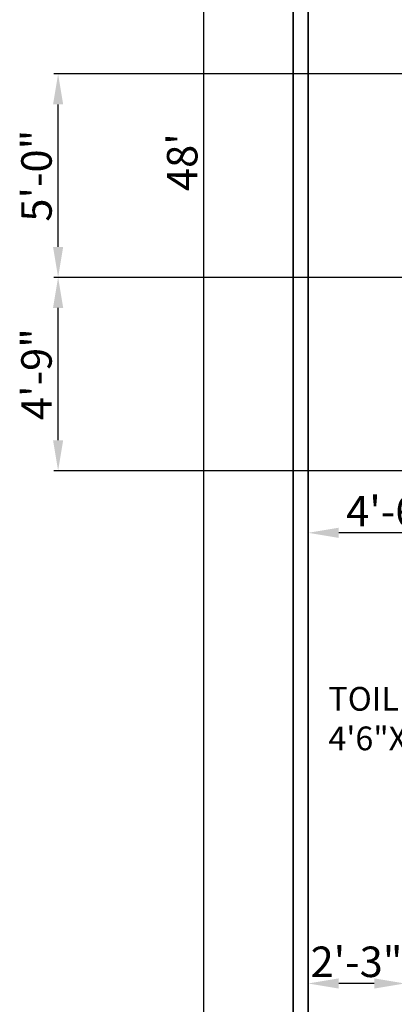
# Model space of a CAD drawing. Units: inches. Extents: x 53662 to 54269, y 37303 to 38048.
# Tile 2 of 6: x 53669 to 53780, y 37459 to 37749. Entities that reach past the tile are written whole.
import ezdxf

# ---------------------------------------------------------------- set-up
doc = ezdxf.new("R2010")
doc.units = ezdxf.units.IN
for name, color, linetype, lineweight in [('A-ANNO-DIMS', 2, 'Continuous', 18), ('A-AREA-IDEN', 7, 'Continuous', 25), ('C-PROP', 7, 'Continuous', 35)]:
    doc.layers.add(name, color=color, linetype=linetype, lineweight=lineweight)
doc.styles.get("Standard").update_dxf_attribs({"font": 'arial.ttf'})
doc.dimstyles.new('ISO-25', dxfattribs={"dimtxt": 9, "dimasz": 9, "dimexe": 1.25, "dimexo": 0.625, "dimtad": 1, "dimdec": 1, "dimrnd": 9, "dimlunit": 3, "dimtxsty": 'Standard', "dimcen": 2.5, "dimadec": 0, "dimazin": 0, "dimtfac": 1, "dimtdec": 1, "dimtmove": 0, "dimatfit": 3, "dimfxl": 1, "dimarcsym": 0})

# ---------------------------------------------------------------- blocks, each defined once
blk = doc.blocks.new('*D13')
at = {"layer": 'A-ANNO-DIMS', "color": 0, "lineweight": -2, "transparency": 16777216}
for p, q in [((53749.49, 37994.86), (53722.52, 37994.86)), ((53723.77, 37427.86), (53723.77, 37985.86)), ((53749.49, 37418.86), (53722.52, 37418.86))]:
    blk.add_line(p, q, dxfattribs=at)
at = {"layer": 'A-ANNO-DIMS', "color": 0, "transparency": 16777216}
for points in [[(53722.27, 37985.86), (53725.27, 37985.86), (53723.77, 37994.86)], [(53722.27, 37427.86), (53725.27, 37427.86), (53723.77, 37418.86)]]:
    blk.add_solid(points, dxfattribs=at)
at = {"layer": 'Defpoints', "color": 0, "transparency": 16777216}
for p in [(53723.77, 37994.86), (53750.11, 37994.86), (53750.11, 37418.86)]:
    blk.add_point(p, dxfattribs=at)
at = {"layer": 'A-ANNO-DIMS', "color": 0, "transparency": 16777216, "insert": (53718.55, 37706.86), "char_height": 9, "attachment_point": 5, "rotation": 90}
blk.add_mtext("48'", dxfattribs=at)
blk = doc.blocks.new('*D15')
at = {"layer": 'A-ANNO-DIMS', "color": 0, "lineweight": -2, "transparency": 16777216}
for p, q in [((53754.61, 37615.24), (53754.61, 37596.31)), ((53804.11, 37615.24), (53804.11, 37596.31)), ((53795.11, 37597.56), (53763.61, 37597.56))]:
    blk.add_line(p, q, dxfattribs=at)
at = {"layer": 'A-ANNO-DIMS', "color": 0, "transparency": 16777216}
for points in [[(53763.61, 37599.06), (53763.61, 37596.06), (53754.61, 37597.56)], [(53795.11, 37599.06), (53795.11, 37596.06), (53804.11, 37597.56)]]:
    blk.add_solid(points, dxfattribs=at)
at = {"layer": 'Defpoints', "color": 0, "transparency": 16777216}
for p in [(53754.61, 37615.86), (53804.11, 37615.86), (53754.61, 37597.56)]:
    blk.add_point(p, dxfattribs=at)
at = {"layer": 'A-ANNO-DIMS', "color": 0, "transparency": 16777216, "insert": (53779.36, 37602.78), "char_height": 9, "attachment_point": 5}
blk.add_mtext('4\'-6"', dxfattribs=at)
blk = doc.blocks.new('*D17')
at = {"layer": 'A-ANNO-DIMS', "color": 0, "lineweight": -2, "transparency": 16777216}
for p, q in [((53754.61, 37463.49), (53754.61, 37465.93)), ((53783.11, 37463.49), (53783.11, 37465.93)), ((53774.11, 37464.68), (53763.61, 37464.68))]:
    blk.add_line(p, q, dxfattribs=at)
at = {"layer": 'A-ANNO-DIMS', "color": 0, "transparency": 16777216}
for points in [[(53763.61, 37466.18), (53763.61, 37463.18), (53754.61, 37464.68)], [(53774.11, 37466.18), (53774.11, 37463.18), (53783.11, 37464.68)]]:
    blk.add_solid(points, dxfattribs=at)
at = {"layer": 'Defpoints', "color": 0, "transparency": 16777216}
for p in [(53754.61, 37464.68), (53754.61, 37462.86), (53783.11, 37462.86)]:
    blk.add_point(p, dxfattribs=at)
at = {"layer": 'A-ANNO-DIMS', "color": 0, "transparency": 16777216, "insert": (53768.86, 37469.9), "char_height": 9, "attachment_point": 5}
blk.add_mtext('2\'-3"', dxfattribs=at)
blk = doc.blocks.new('*D64')
at = {"layer": 'A-ANNO-DIMS', "color": 0, "lineweight": -2, "transparency": 16777216}
for p, q in [((53782.49, 37672.86), (53679.5, 37672.86)), ((53680.75, 37624.86), (53680.75, 37663.86)), ((53782.49, 37615.86), (53679.5, 37615.86))]:
    blk.add_line(p, q, dxfattribs=at)
at = {"layer": 'A-ANNO-DIMS', "color": 0, "transparency": 16777216}
for points in [[(53679.25, 37663.86), (53682.25, 37663.86), (53680.75, 37672.86)], [(53679.25, 37624.86), (53682.25, 37624.86), (53680.75, 37615.86)]]:
    blk.add_solid(points, dxfattribs=at)
at = {"layer": 'Defpoints', "color": 0, "transparency": 16777216}
for p in [(53680.75, 37672.86), (53783.11, 37672.86), (53783.11, 37615.86)]:
    blk.add_point(p, dxfattribs=at)
at = {"layer": 'A-ANNO-DIMS', "color": 0, "transparency": 16777216, "insert": (53675.53, 37644.36), "char_height": 9, "attachment_point": 5, "rotation": 90}
blk.add_mtext('4\'-9"', dxfattribs=at)
blk = doc.blocks.new('*D65')
at = {"layer": 'A-ANNO-DIMS', "color": 0, "lineweight": -2, "transparency": 16777216}
for p, q in [((53782.49, 37732.86), (53679.5, 37732.86)), ((53680.75, 37681.86), (53680.75, 37723.86)), ((53782.49, 37672.86), (53679.5, 37672.86))]:
    blk.add_line(p, q, dxfattribs=at)
at = {"layer": 'A-ANNO-DIMS', "color": 0, "transparency": 16777216}
for points in [[(53679.25, 37723.86), (53682.25, 37723.86), (53680.75, 37732.86)], [(53679.25, 37681.86), (53682.25, 37681.86), (53680.75, 37672.86)]]:
    blk.add_solid(points, dxfattribs=at)
at = {"layer": 'Defpoints', "color": 0, "transparency": 16777216}
for p in [(53680.75, 37732.86), (53783.11, 37732.86), (53783.11, 37672.86)]:
    blk.add_point(p, dxfattribs=at)
at = {"layer": 'A-ANNO-DIMS', "color": 0, "transparency": 16777216, "insert": (53675.53, 37702.86), "char_height": 9, "attachment_point": 5, "rotation": 90}
blk.add_mtext('5\'-0"', dxfattribs=at)

msp = doc.modelspace()

# ---------------------------------------------------------------- linework, layer by layer
at = {"layer": 'C-PROP'}
for p, q in [((53750.11, 37994.86), (53750.11, 37615.86)), ((53754.61, 37990.36), (53754.61, 37615.86)), ((53750.11, 37418.86), (53750.11, 37615.86)), ((53754.61, 37423.36), (53754.61, 37615.86))]:
    msp.add_line(p, q, dxfattribs=at)

# ---------------------------------------------------------------- texts
at = {"layer": 'A-AREA-IDEN', "insert": (53760.56, 37552.11), "char_height": 7, "attachment_point": 1}
msp.add_mtext_dynamic_manual_height_columns('TOILET\\P4\'6"X8\'0"', width=40.1945, gutter_width=12.5, heights=[0], dxfattribs=at)

# ---------------------------------------------------------------- dimensions: what is measured, and where the dimension line sits
at = {"layer": 'A-ANNO-DIMS'}
for base, p1, p2, override, picture, middle in [((53723.77, 37994.86), (53750.11, 37418.86), (53750.11, 37994.86), {"dimclrd": 0, "dimclre": 0, "dimclrt": 0}, '*D13', (53718.55, 37706.86)), ((53680.75, 37732.86), (53783.11, 37672.86), (53783.11, 37732.86), {"dimdec": 1, "dimlfac": 1, "dimrnd": 0, "dimzin": 1, "dimdsep": 46, "dimlunit": 4, "dimfrac": 2}, '*D65', (53675.53, 37702.86)), ((53680.75, 37672.86), (53783.11, 37615.86), (53783.11, 37672.86), {"dimdec": 1, "dimlfac": 1, "dimrnd": 0, "dimzin": 1, "dimdsep": 46, "dimlunit": 4, "dimfrac": 2}, '*D64', (53675.53, 37644.36))]:
    dim = msp.add_linear_dim(base=base, p1=p1, p2=p2, angle=90, dimstyle='ISO-25', override=override, dxfattribs=at)
    dim.commit()
    dim.dimension.update_dxf_attribs({"geometry": picture, "text_midpoint": middle})
for base, p1, p2, picture, middle in [((53754.61, 37597.56), (53804.11, 37615.86), (53754.61, 37615.86), '*D15', (53779.36, 37602.78)), ((53754.61, 37464.68), (53783.11, 37462.86), (53754.61, 37462.86), '*D17', (53768.86, 37469.9))]:
    dim = msp.add_linear_dim(base=base, p1=p1, p2=p2, dimstyle='ISO-25', override={"dimclrd": 0, "dimclre": 0, "dimclrt": 0}, dxfattribs=at)
    dim.commit()
    dim.dimension.update_dxf_attribs({"geometry": picture, "text_midpoint": middle})

doc.saveas('drawing.dxf')
